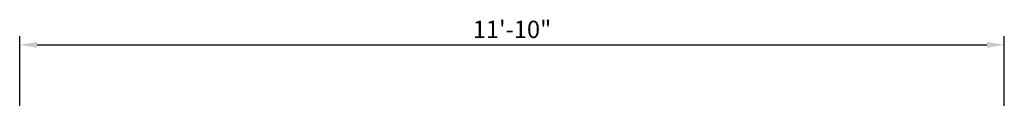
# Model space of a CAD drawing. Units: inches. Extents: x 457 to 882, y 0 to 1111.
# Tile 1 of 4: x 700 to 842, y 0 to 13. Entities that reach past the tile are written whole.
import ezdxf

# ---------------------------------------------------------------- set-up
doc = ezdxf.new("R2010")
doc.units = ezdxf.units.IN
doc.layers.add('A-ANNO-DIMS', color=2, linetype='Continuous', lineweight=18)
doc.styles.get("Standard").update_dxf_attribs({"font": 'arial.ttf'})
doc.dimstyles.new('ISO-25', dxfattribs={"dimtxt": 2.5, "dimasz": 2.5, "dimexe": 1.25, "dimexo": 0.625, "dimtad": 1, "dimdec": 0, "dimlunit": 3, "dimtxsty": 'Standard', "dimcen": 2.5, "dimadec": 0, "dimazin": 0, "dimtfac": 1, "dimtdec": 0, "dimtmove": 0, "dimatfit": 3, "dimfxl": 1, "dimarcsym": 0})

# ---------------------------------------------------------------- blocks, each defined once
blk = doc.blocks.new('*D4')
at = {"layer": 'A-ANNO-DIMS', "color": 0, "lineweight": -2, "transparency": 16777216}
for p, q in [((700.26, 0.62), (700.26, 10.66)), ((842.26, 0.62), (842.26, 10.66)), ((702.76, 9.41), (839.76, 9.41))]:
    blk.add_line(p, q, dxfattribs=at)
at = {"layer": 'A-ANNO-DIMS', "color": 0, "transparency": 16777216}
for points in [[(702.76, 9.83), (702.76, 8.99), (700.26, 9.41)], [(839.76, 9.83), (839.76, 8.99), (842.26, 9.41)]]:
    blk.add_solid(points, dxfattribs=at)
at = {"layer": 'Defpoints', "color": 0, "transparency": 16777216}
for p in [(842.26, 9.41), (700.26, 0), (842.26, 0)]:
    blk.add_point(p, dxfattribs=at)
at = {"layer": 'A-ANNO-DIMS', "color": 0, "transparency": 16777216, "insert": (771.26, 11.31), "char_height": 2.5, "attachment_point": 5}
blk.add_mtext('11\'-10"', dxfattribs=at)

msp = doc.modelspace()

# ---------------------------------------------------------------- dimensions: what is measured, and where the dimension line sits
at = {"layer": 'A-ANNO-DIMS'}
dim = msp.add_linear_dim(base=(842.26, 9.41), p1=(700.26, 0), p2=(842.26, 0), dimstyle='ISO-25', override={"dimclrd": 0, "dimclre": 0, "dimclrt": 0}, dxfattribs=at)
dim.commit()
dim.dimension.update_dxf_attribs({"geometry": '*D4', "text_midpoint": (771.26, 11.31)})

doc.saveas('drawing.dxf')
